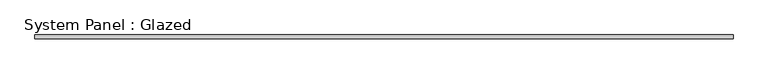
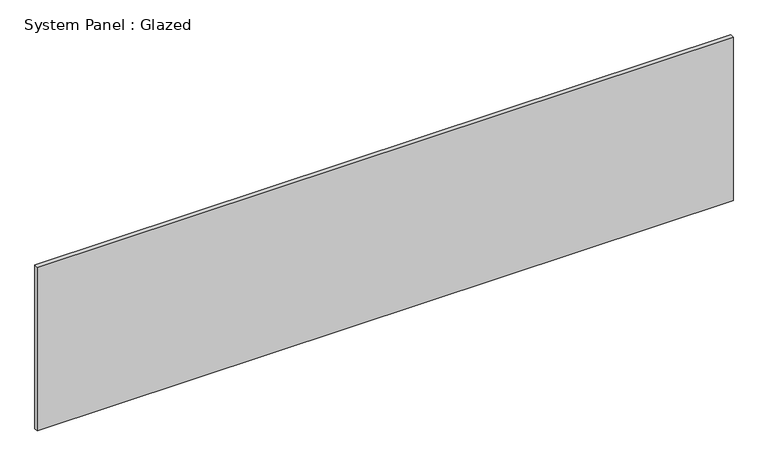
"""IFC4 building model written with IfcOpenShell, lengths in millimetres: plate geometry, System Panel : Glazed."""

from ifc_helpers import new_model, si_unit, origin, origin_with_axes, place, context, project, spatial, polyline, outline, extrude, source, transform, mapped, element, save


def system_panel_glazed_7fa16c81(model_context):
    return source(origin(), model_context, "Body", "SweptSolid", [
        extrude(outline(polyline([(2323.1452201, 19.05), (-2323.1452201, 19.05), (-2323.1452201, 44.45), (2323.1452201, 44.45), (2323.1452201, 19.05)])), origin_with_axes(), (0.0, 0.0, 1.0), 1155.7),
    ])


if __name__ == "__main__":
    model = new_model("IFC4")
    model_context = context("Model", 3, world=origin())
    ifc_project = project(units=[si_unit("LENGTHUNIT", "METRE", prefix="MILLI")], contexts=[model_context])
    site = spatial("IfcSite", under=ifc_project)
    building = spatial("IfcBuilding", under=site)
    placement = place(None, origin())
    system_panel_glazed_shape = system_panel_glazed_7fa16c81(model_context)
    element("IfcPlate", 1, ObjectType="System Panel : Glazed", at=placement, inside=building, context=model_context, shape_type="MappedRepresentation", body=[
        mapped(system_panel_glazed_shape, transform((0.0, 0.0, 0.0), x_axis=(1.0, 0.0, 0.0), y_axis=(0.0, 1.0, 0.0), z_axis=(0.0, 0.0, 1.0))),
    ])
    save(model, "model.ifc")

# Revit data of these elements
# Type "System Panel : Glazed"
#   Construction Type Id = "GSP4R"
#   Analytic Construction = "1/8 in Pilkington single glazing"
#   Visual Light Transmittance = 0.9
#   Solar Heat Gain Coefficient = 0.86
#   Heat Transfer Coefficient (U) = 1.18115 BTU/(h·ft²·°F)
# Element 1 (IfcPlate, "System Panel : Glazed")
#   Materials on its faces: "Glass"
# Materials
#   "Glass": class "Glass", colour RGB 0 128 192, transparency 0.75, Description = "Soda Lime Glass", Cost = 0
